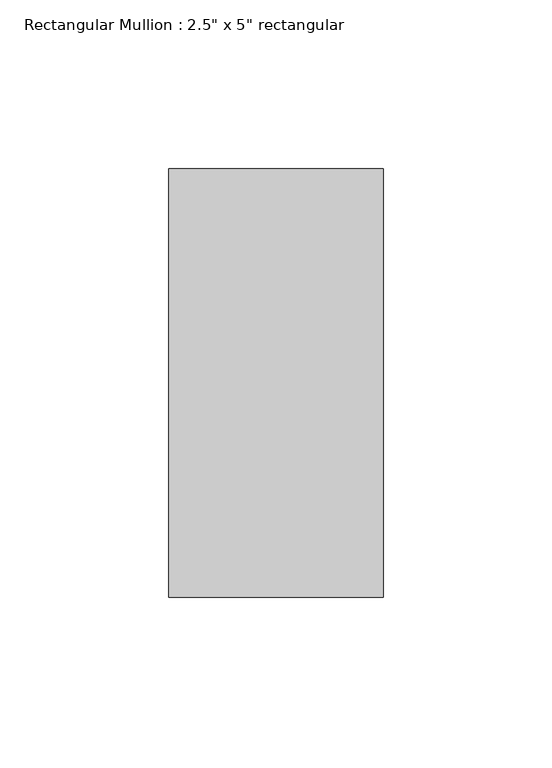
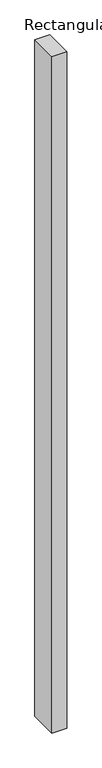
"""IFC4 building model written with IfcOpenShell, lengths in millimetres: member geometry."""

from ifc_helpers import new_model, si_unit, frame, origin, place, context, project, spatial, polyline, outline, extrude, source, transform, mapped, element, save


def member_3783eaa0(model_context):
    return source(origin(), model_context, "Body", "SweptSolid", [
        extrude(outline(polyline([(0.0, 63.5), (0.0, -63.5), (-63.5, -63.5), (-63.5, 63.5), (0.0, 63.5)])), frame((0.0, 0.0, -3073.4), z_axis=(0.0, 0.0, 1.0), x_axis=(1.0, 0.0, 0.0)), (0.0, 0.0, 1.0), 3073.4),
    ])


if __name__ == "__main__":
    model = new_model("IFC4")
    model_context = context("Model", 3, world=origin())
    ifc_project = project(units=[si_unit("LENGTHUNIT", "METRE", prefix="MILLI")], contexts=[model_context])
    site = spatial("IfcSite", under=ifc_project)
    building = spatial("IfcBuilding", under=site)
    placement = place(None, origin())
    member_shape = member_3783eaa0(model_context)
    element("IfcMember", 1, ObjectType="Rectangular Mullion : 2.5\" x 5\" rectangular", at=placement, inside=building, context=model_context, shape_type="MappedRepresentation", body=[
        mapped(member_shape, transform((0.0, 0.0, 0.0), x_axis=(1.0, 0.0, 0.0), y_axis=(0.0, 1.0, 0.0), z_axis=(0.0, 0.0, 1.0))),
    ])
    save(model, "model.ifc")

# Revit data of these elements
# Type "Rectangular Mullion : 2.5\" x 5\" rectangular"
#   built-in parameter 1007304 = 0.416667 (stored number, unit not read)
#   built-in parameter 1007301 = 0.104167 (stored number, unit not read)
#   built-in parameter 1007300 = 0.104167 (stored number, unit not read)
# Element 1 (IfcMember, "Rectangular Mullion : 2.5\" x 5\" rectangular")
#   Materials on its faces: "Iron, Ductile"
# Materials
#   "Iron, Ductile": class "Metal", colour RGB 0 0 0, transparency 0, Description = "Ductile cast iron", Cost = 0
